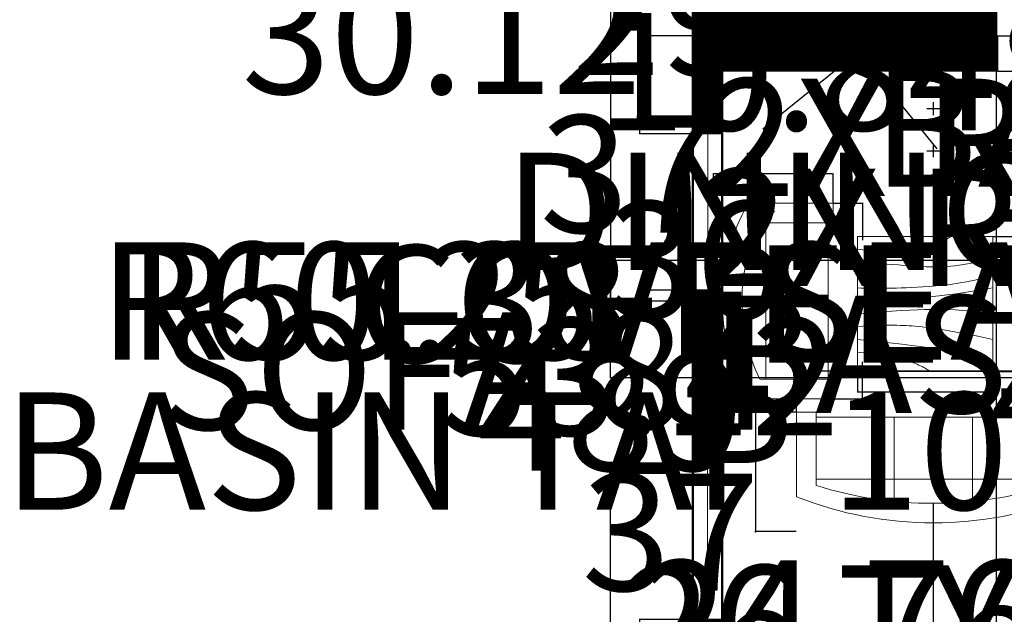
# Model space of a CAD drawing. Units: inches. Extents: x 1173 to 2157, y 515 to 1129.
# Tile 2 of 13: x 1173 to 1475, y 747 to 929. Entities that reach past the tile are written whole.
import ezdxf

# ---------------------------------------------------------------- set-up
doc = ezdxf.new("R2010")
doc.units = ezdxf.units.IN
doc.header["$MEASUREMENT"] = 0
for name, color, linetype, lineweight in [('A-ANNO-DIMS', 2, 'Continuous', 18), ('A-FLOR-CASE', 32, 'Continuous', 25), ('A-FURN', 8, 'Continuous', 18), ('A-GLAZ', 4, 'Continuous', 18), ('A-WALL', 7, 'Continuous', 50)]:
    doc.layers.add(name, color=color, linetype=linetype, lineweight=lineweight)
doc.layers.add('A-FLOR-CASE-PATT', color=28, linetype='Continuous', lineweight=13, true_color=0x301203)
doc.layers.add('A-WALL-PATT', color=22, linetype='Continuous', lineweight=13, true_color=0xca4b0c)
doc.styles.get("Standard").update_dxf_attribs({"font": 'arial.ttf'})
doc.dimstyles.get("Standard").update_dxf_attribs({"dimtxt": 36, "dimasz": 0.18, "dimexe": 0.18, "dimexo": 0.0625, "dimgap": 0.09, "dimtad": 0, "dimtih": 1, "dimtoh": 1, "dimdec": 0, "dimrnd": 72, "dimzin": 0, "dimdsep": 46, "dimlunit": 3, "dimtxsty": 'Standard', "dimcen": 2, "dimadec": 0, "dimazin": 0, "dimtfac": 1, "dimtdec": 0, "dimtofl": 0, "dimtmove": 0, "dimatfit": 3, "dimfxl": 1, "dimtolj": 1, "dimtzin": 0, "dimarcsym": 0})

# ---------------------------------------------------------------- blocks, each defined once
blk = doc.blocks.new('Table - Square Woodgrain 42 x 42 in.')
blk.add_line((0, -42), (42, -42))
for points in [[(0, -4), (1.704, -4.2172), (3.2358, -4.4188), (4.615, -4.604), (5.8615, -4.7721), (6.9951, -4.9224), (8.0357, -5.0541), (9.0031, -5.1667), (9.9171, -5.2594), (10.7951, -5.3316), (11.6445, -5.3836), (12.4702, -5.4157), (13.277, -5.4283), (14.0698, -5.4217), (14.8535, -5.3964), (15.6331, -5.3526), (16.4133, -5.2908), (17.1986, -5.2103), (17.9913, -5.1062), (18.793, -4.9727), (19.6056, -4.8038), (20.4307, -4.5937), (21.2701, -4.3365), (22.1256, -4.0262), (22.9989, -3.6571), (23.888, -3.2272), (24.7756, -2.7516), (25.6408, -2.2491), (26.4624, -1.7387), (27.2195, -1.2395), (27.891, -0.7703), (28.456, -0.3501), (28.8934, 0.002)], [(0, -42), (0, 0), (42, 0), (42, -42)], [(0, -8), (1.8203, -8.1001), (3.6741, -8.2149), (5.5411, -8.3408), (7.4011, -8.4741), (9.2339, -8.6112), (11.0193, -8.7484), (12.7371, -8.8821), (14.3671, -9.0086), (15.8954, -9.1246), (17.3337, -9.2278), (18.6997, -9.3159), (20.0116, -9.387), (21.2871, -9.4389), (22.5442, -9.4696), (23.8008, -9.477), (25.0749, -9.459), (26.3791, -9.4137), (27.7049, -9.3403), (29.0383, -9.2382), (30.3655, -9.1068), (31.6728, -8.9455), (32.9461, -8.7535), (34.1717, -8.5304), (35.3358, -8.2756), (36.4268, -7.9863), (37.443, -7.6521), (38.3849, -7.2603), (39.253, -6.7986), (40.048, -6.2542), (40.7705, -5.6147), (41.421, -4.8674), (42, -4)], [(42, -12), (39.1784, -12.8621), (36.4519, -13.5654), (33.8246, -14.1294), (31.3004, -14.5731), (28.8832, -14.9161), (26.577, -15.1775), (24.3858, -15.3768), (22.3136, -15.5332), (20.3622, -15.6632), (18.5254, -15.7718), (16.7947, -15.8612), (15.1618, -15.9338), (13.6183, -15.9916), (12.1558, -16.0369), (10.7659, -16.0718), (9.4403, -16.0987), (8.1703, -16.1191), (6.9461, -16.1325), (5.7577, -16.1377), (4.595, -16.1335), (3.4479, -16.1188), (2.3064, -16.0924), (1.1604, -16.0532), (0, -16)], [(42, -16), (37.6529, -16.7365), (33.8802, -17.329), (30.6179, -17.7961), (27.8015, -18.1561), (25.3668, -18.4275), (23.2497, -18.6288), (21.3859, -18.7785), (19.7111, -18.8949), (18.1693, -18.9939), (16.7375, -19.0795), (15.401, -19.1534), (14.1449, -19.217), (12.9544, -19.2717), (11.8148, -19.3191), (10.7113, -19.3606), (9.6291, -19.3976), (8.5534, -19.4323), (7.47, -19.4689), (6.3643, -19.5122), (5.222, -19.5672), (4.0288, -19.6386), (2.7703, -19.7313), (1.4321, -19.8501), (0, -20)], [(0, -24), (3.9243, -23.6805), (7.4766, -23.4138), (10.6891, -23.1954), (13.5943, -23.0205), (16.2247, -22.8847), (18.6125, -22.7832), (20.7903, -22.7116), (22.7903, -22.6651), (24.6563, -22.642), (26.4764, -22.6507), (28.35, -22.7024), (30.3766, -22.8084), (32.6555, -22.98), (35.2861, -23.2283), (38.3678, -23.5645), (42, -24)], [(42, -32), (37.392, -31.017), (33.4585, -30.2231), (30.1291, -29.5949), (27.3334, -29.109), (25.0009, -28.742), (23.0612, -28.4707), (21.4439, -28.2716), (20.0786, -28.1215), (18.8998, -28.0002), (17.8609, -27.9014), (16.9206, -27.8219), (16.0371, -27.7588), (15.1691, -27.709), (14.2748, -27.6693), (13.3128, -27.6368), (12.2415, -27.6083), (11.0295, -27.5824), (9.6867, -27.5643), (8.233, -27.5608), (6.6884, -27.5787), (5.0728, -27.6248), (3.4062, -27.7058), (1.7086, -27.8286), (0, -28)], [(0, -32), (5.4026, -32.5358), (9.9494, -33.019), (13.7424, -33.4553), (16.8834, -33.8505), (19.4743, -34.2106), (21.6171, -34.5413), (23.4136, -34.8486), (24.9657, -35.1382), (26.3614, -35.4156), (27.6332, -35.6841), (28.7995, -35.9467), (29.8788, -36.2064), (30.8897, -36.4661), (31.8507, -36.7288), (32.7802, -36.9973), (33.6968, -37.2747), (34.6175, -37.5635), (35.5531, -37.8651), (36.5128, -38.1805), (37.506, -38.5108), (38.5421, -38.8568), (39.6302, -39.2197), (40.7797, -39.6004), (42, -40)], [(0, -36), (3.0098, -36.2857), (5.5354, -36.5643), (7.6368, -36.8359), (9.374, -37.1009), (10.807, -37.3597), (11.9957, -37.6126), (13.0002, -37.8599), (13.8804, -38.102), (14.6874, -38.3393), (15.4365, -38.5729), (16.1338, -38.8041), (16.7858, -39.0341), (17.3987, -39.264), (17.9787, -39.4952), (18.5322, -39.7288), (19.0655, -39.9662), (19.5832, -40.2081), (20.0842, -40.4544), (20.5657, -40.7046), (21.0249, -40.9581), (21.459, -41.2144), (21.8653, -41.4731), (22.2409, -41.7335), (22.5831, -41.9951)]]:
    blk.add_lwpolyline(points)
blk = doc.blocks.new('Sofa - Roundback Loveseat 5 ft.')
for p, q in [((0, -32.44198), (0, -5.99998)), ((-24, -33.99998), (-24, -11.46958)), ((24.00004, -33.99998), (24.00004, -11.46958)), ((-23.9998, -13.38178), (23.99986, -13.38178)), ((-24, -32.44198), (24.00004, -32.44198))]:
    blk.add_line(p, q)
for points in [[(-24, -33.99998), (-30, -33.99998), (-30, -7.99998)], [(30.00004, -7.99998), (30.00004, -33.99998), (24.00004, -33.99998)]]:
    blk.add_lwpolyline(points)
for centre, radius, start, end in [((0, -60.24998), 60.24998, 60.13715, 119.8628), ((0, -61.38438), 55.38444, 64.32083, 115.6792)]:
    blk.add_arc(centre, radius, start, end)
blk = doc.blocks.new('Sofa - Roundback 7 ft.')
for p, q in [((-12.00002, -32.4421), (-12.00003, -6.5971)), ((11.99997, -32.4421), (11.99998, -6.5971)), ((-36.000027, -34), (-36.000027, -11.4696)), ((35.99998, -34), (35.99998, -11.4696)), ((-35.999844, -13.3819), (35.9998, -13.3819)), ((-36.000027, -32.4421), (35.99998, -32.4421))]:
    blk.add_line(p, q)
for points in [[(-36.000027, -34), (-42.000027, -34), (-42.000027, -8)], [(41.99998, -8), (41.99998, -34), (35.99998, -34)]]:
    blk.add_lwpolyline(points)
for centre, radius, start, end in [((0, -114.25), 114.25, 68.43141, 111.5686), ((-0.00001, -127.1968), 121.1968, 72.72033, 107.2797)]:
    blk.add_arc(centre, radius, start, end)
blk = doc.blocks.new('WIN-48X9')
blk.add_line((48, 4.5), (0, 4.5))
blk.add_lwpolyline([(0, 9), (48, 9), (48, 0), (0, 0)], close=True)
blk = doc.blocks.new('*D30')
at = {"layer": 'A-ANNO-DIMS', "color": 0, "lineweight": -2, "transparency": 16777216}
for p, q in [((1555.97, 736.03), (1563.78, 736.03)), ((1563.6, 735.85), (1563.6, 729.12)), ((1563.6, 684.97), (1563.6, 691.71)), ((1555.97, 684.79), (1563.78, 684.79))]:
    blk.add_line(p, q, dxfattribs=at)
at = {"layer": 'A-ANNO-DIMS', "color": 0, "transparency": 16777216}
for points in [[(1563.57, 735.85), (1563.63, 735.85), (1563.6, 736.03)], [(1563.57, 684.97), (1563.63, 684.97), (1563.6, 684.79)]]:
    blk.add_solid(points, dxfattribs=at)
at = {"layer": 'Defpoints', "color": 0, "transparency": 16777216}
for p in [(1555.91, 736.03), (1563.6, 736.03), (1555.91, 684.79)]:
    blk.add_point(p, dxfattribs=at)
at = {"layer": 'A-ANNO-DIMS', "color": 0, "transparency": 16777216, "insert": (1563.6, 710.41), "char_height": 36, "attachment_point": 5}
blk.add_mtext('\\A1;DESK 51 TYP.', dxfattribs=at)
blk = doc.blocks.new('*D31')
at = {"layer": 'A-ANNO-DIMS', "color": 0, "lineweight": -2, "transparency": 16777216}
for p, q in [((1529.44, 743.72), (1529.26, 743.72)), ((1529.44, 736.09), (1529.44, 743.9)), ((1555.73, 743.72), (1529.62, 743.72)), ((1555.91, 736.09), (1555.91, 743.9))]:
    blk.add_line(p, q, dxfattribs=at)
at = {"layer": 'A-ANNO-DIMS', "color": 0, "transparency": 16777216}
for points in [[(1529.62, 743.75), (1529.62, 743.69), (1529.44, 743.72)], [(1555.73, 743.75), (1555.73, 743.69), (1555.91, 743.72)]]:
    blk.add_solid(points, dxfattribs=at)
at = {"layer": 'Defpoints', "color": 0, "transparency": 16777216}
for p in [(1529.44, 743.72), (1529.44, 736.03), (1555.91, 736.03)]:
    blk.add_point(p, dxfattribs=at)
at = {"layer": 'A-ANNO-DIMS', "color": 0, "transparency": 16777216, "insert": (1441.24, 743.72), "char_height": 36, "attachment_point": 5}
blk.add_mtext('\\A1;26 TYP.', dxfattribs=at)
blk = doc.blocks.new('*D36')
at = {"layer": 'A-ANNO-DIMS', "color": 0, "lineweight": -2, "transparency": 16777216}
for p, q in [((1497.87, 905.02), (1487.37, 905.02)), ((1487.55, 904.84), (1487.55, 889.09)), ((1487.55, 835.93), (1487.55, 851.68)), ((1497.87, 835.75), (1487.37, 835.75))]:
    blk.add_line(p, q, dxfattribs=at)
at = {"layer": 'A-ANNO-DIMS', "color": 0, "transparency": 16777216}
for points in [[(1487.52, 904.84), (1487.58, 904.84), (1487.55, 905.02)], [(1487.52, 835.93), (1487.58, 835.93), (1487.55, 835.75)]]:
    blk.add_solid(points, dxfattribs=at)
at = {"layer": 'Defpoints', "color": 0, "transparency": 16777216}
for p in [(1497.94, 905.02), (1487.55, 835.75), (1497.94, 835.75)]:
    blk.add_point(p, dxfattribs=at)
at = {"layer": 'A-ANNO-DIMS', "color": 0, "transparency": 16777216, "insert": (1487.55, 870.38), "char_height": 36, "attachment_point": 5}
blk.add_mtext('\\A1;DINING SET 69', dxfattribs=at)
blk = doc.blocks.new('*D38')
at = {"layer": 'A-ANNO-DIMS', "color": 0, "lineweight": -2, "transparency": 16777216}
for p, q in [((1471.69, 862.7), (1478.04, 862.7)), ((1477.86, 862.52), (1477.86, 860.65)), ((1477.86, 821.35), (1477.86, 823.22)), ((1471.69, 821.17), (1478.04, 821.17))]:
    blk.add_line(p, q, dxfattribs=at)
at = {"layer": 'A-ANNO-DIMS', "color": 0, "transparency": 16777216}
for points in [[(1477.83, 862.52), (1477.89, 862.52), (1477.86, 862.7)], [(1477.83, 821.35), (1477.89, 821.35), (1477.86, 821.17)]]:
    blk.add_solid(points, dxfattribs=at)
at = {"layer": 'Defpoints', "color": 0, "transparency": 16777216}
for p in [(1471.63, 862.7), (1477.86, 862.7), (1471.63, 821.17)]:
    blk.add_point(p, dxfattribs=at)
at = {"layer": 'A-ANNO-DIMS', "color": 0, "transparency": 16777216, "insert": (1477.86, 841.93), "char_height": 36, "attachment_point": 5}
blk.add_mtext('\\A1;COFFEE TABLE 42', dxfattribs=at)
blk = doc.blocks.new('*D39')
at = {"layer": 'A-ANNO-DIMS', "color": 0, "lineweight": -2, "transparency": 16777216}
for p, q in [((1430.11, 821.11), (1430.11, 814.76)), ((1471.63, 821.11), (1471.63, 814.76)), ((1430.29, 814.94), (1471.45, 814.94)), ((1471.63, 814.94), (1471.81, 814.94))]:
    blk.add_line(p, q, dxfattribs=at)
at = {"layer": 'A-ANNO-DIMS', "color": 0, "transparency": 16777216}
for points in [[(1430.29, 814.97), (1430.29, 814.91), (1430.11, 814.94)], [(1471.45, 814.97), (1471.45, 814.91), (1471.63, 814.94)]]:
    blk.add_solid(points, dxfattribs=at)
at = {"layer": 'Defpoints', "color": 0, "transparency": 16777216}
for p in [(1430.11, 821.17), (1471.63, 821.17), (1471.63, 814.94)]:
    blk.add_point(p, dxfattribs=at)
at = {"layer": 'A-ANNO-DIMS', "color": 0, "transparency": 16777216, "insert": (1498.22, 814.94), "char_height": 36, "attachment_point": 5}
blk.add_mtext('\\A1;42', dxfattribs=at)
blk = doc.blocks.new('*D40')
at = {"layer": 'A-ANNO-DIMS', "color": 0, "lineweight": -2, "transparency": 16777216}
for p, q in [((1422.73, 872.86), (1431.84, 872.86)), ((1431.66, 872.68), (1431.66, 861.58)), ((1431.66, 813.04), (1431.66, 824.15)), ((1422.73, 812.86), (1431.84, 812.86))]:
    blk.add_line(p, q, dxfattribs=at)
at = {"layer": 'A-ANNO-DIMS', "color": 0, "transparency": 16777216}
for points in [[(1431.63, 872.68), (1431.69, 872.68), (1431.66, 872.86)], [(1431.63, 813.04), (1431.69, 813.04), (1431.66, 812.86)]]:
    blk.add_solid(points, dxfattribs=at)
at = {"layer": 'Defpoints', "color": 0, "transparency": 16777216}
for p in [(1422.66, 872.86), (1431.66, 872.86), (1422.66, 812.86)]:
    blk.add_point(p, dxfattribs=at)
at = {"layer": 'A-ANNO-DIMS', "color": 0, "transparency": 16777216, "insert": (1431.66, 842.86), "char_height": 36, "attachment_point": 5}
blk.add_mtext('\\A1;LOVESEAT 60', dxfattribs=at)
blk = doc.blocks.new('*D41')
at = {"layer": 'A-ANNO-DIMS', "color": 0, "lineweight": -2, "transparency": 16777216}
for p, q in [((1386, 872.92), (1386, 882.04)), ((1422.66, 872.92), (1422.66, 882.04)), ((1386, 881.86), (1385.82, 881.86)), ((1422.48, 881.86), (1386.18, 881.86))]:
    blk.add_line(p, q, dxfattribs=at)
at = {"layer": 'A-ANNO-DIMS', "color": 0, "transparency": 16777216}
for points in [[(1386.18, 881.89), (1386.18, 881.83), (1386, 881.86)], [(1422.48, 881.89), (1422.48, 881.83), (1422.66, 881.86)]]:
    blk.add_solid(points, dxfattribs=at)
at = {"layer": 'Defpoints', "color": 0, "transparency": 16777216}
for p in [(1386, 881.86), (1386, 872.86), (1422.66, 872.86)]:
    blk.add_point(p, dxfattribs=at)
at = {"layer": 'A-ANNO-DIMS', "color": 0, "transparency": 16777216, "insert": (1359.95, 881.86), "char_height": 36, "attachment_point": 5}
blk.add_mtext('\\A1;37', dxfattribs=at)
blk = doc.blocks.new('*D42')
at = {"layer": 'A-ANNO-DIMS', "color": 0, "lineweight": -2, "transparency": 16777216}
for p, q in [((1411.43, 808.8), (1411.43, 821.52)), ((1495.43, 808.8), (1495.43, 821.52)), ((1411.43, 821.34), (1411.25, 821.34)), ((1495.25, 821.34), (1411.61, 821.34))]:
    blk.add_line(p, q, dxfattribs=at)
at = {"layer": 'A-ANNO-DIMS', "color": 0, "transparency": 16777216}
for points in [[(1411.61, 821.37), (1411.61, 821.31), (1411.43, 821.34)], [(1495.25, 821.37), (1495.25, 821.31), (1495.43, 821.34)]]:
    blk.add_solid(points, dxfattribs=at)
at = {"layer": 'Defpoints', "color": 0, "transparency": 16777216}
for p in [(1411.43, 821.34), (1411.43, 808.74), (1495.43, 808.74)]:
    blk.add_point(p, dxfattribs=at)
at = {"layer": 'A-ANNO-DIMS', "color": 0, "transparency": 16777216, "insert": (1310.09, 821.34), "char_height": 36, "attachment_point": 5}
blk.add_mtext('\\A1;SOFA 84', dxfattribs=at)
blk = doc.blocks.new('*D43')
at = {"layer": 'A-ANNO-DIMS', "color": 0, "lineweight": -2, "transparency": 16777216}
for p, q in [((1411.37, 808.74), (1398.65, 808.74)), ((1398.83, 808.56), (1398.83, 772.25)), ((1411.37, 772.07), (1398.65, 772.07)), ((1398.83, 771.89), (1398.65, 771.89)), ((1398.83, 772.07), (1398.83, 771.89))]:
    blk.add_line(p, q, dxfattribs=at)
at = {"layer": 'A-ANNO-DIMS', "color": 0, "transparency": 16777216}
for points in [[(1398.8, 808.56), (1398.86, 808.56), (1398.83, 808.74)], [(1398.8, 772.25), (1398.86, 772.25), (1398.83, 772.07)]]:
    blk.add_solid(points, dxfattribs=at)
at = {"layer": 'Defpoints', "color": 0, "transparency": 16777216}
for p in [(1411.43, 808.74), (1398.83, 772.07), (1411.43, 772.07)]:
    blk.add_point(p, dxfattribs=at)
at = {"layer": 'A-ANNO-DIMS', "color": 0, "transparency": 16777216, "insert": (1372.79, 771.89), "char_height": 36, "attachment_point": 5}
blk.add_mtext('\\A1;37', dxfattribs=at)
blk = doc.blocks.new('*D46')
at = {"layer": 'A-ANNO-DIMS', "color": 0, "lineweight": -2, "transparency": 16777216}
for p, q in [((1648.72, 912.09), (1646.2, 912.17)), ((1646.37, 911.98), (1645.86, 896.32)), ((1645.85, 895.96), (1645.67, 895.96)), ((1648.2, 896.07), (1645.68, 896.15)), ((1645.86, 896.14), (1645.85, 895.96))]:
    blk.add_line(p, q, dxfattribs=at)
at = {"layer": 'A-ANNO-DIMS', "color": 0, "transparency": 16777216}
for points in [[(1646.34, 911.99), (1646.4, 911.98), (1646.38, 912.16)], [(1645.83, 896.32), (1645.89, 896.32), (1645.86, 896.14)]]:
    blk.add_solid(points, dxfattribs=at)
at = {"layer": 'Defpoints', "color": 0, "transparency": 16777216}
for p in [(1648.78, 912.09), (1645.86, 896.14), (1648.26, 896.06)]:
    blk.add_point(p, dxfattribs=at)
at = {"layer": 'A-ANNO-DIMS', "color": 0, "transparency": 16777216, "insert": (1538.16, 895.96), "char_height": 36, "attachment_point": 5}
blk.add_mtext('\\A1;BASIN 16', dxfattribs=at)
blk = doc.blocks.new('*D48')
at = {"layer": 'A-ANNO-DIMS', "color": 0, "lineweight": -2, "transparency": 16777216}
for p, q in [((1592.53, 826.46), (1592.35, 826.47)), ((1592.38, 821.85), (1592.54, 826.64)), ((1623.53, 825.46), (1592.71, 826.46)), ((1623.56, 820.84), (1623.71, 825.64))]:
    blk.add_line(p, q, dxfattribs=at)
at = {"layer": 'A-ANNO-DIMS', "color": 0, "transparency": 16777216}
for points in [[(1592.71, 826.49), (1592.71, 826.43), (1592.53, 826.46)], [(1623.53, 825.49), (1623.53, 825.43), (1623.71, 825.46)]]:
    blk.add_solid(points, dxfattribs=at)
at = {"layer": 'Defpoints', "color": 0, "transparency": 16777216}
for p in [(1592.53, 826.46), (1592.38, 821.79), (1623.56, 820.78)]:
    blk.add_point(p, dxfattribs=at)
at = {"layer": 'A-ANNO-DIMS', "color": 0, "transparency": 16777216, "insert": (1488.3, 826.47), "char_height": 36, "attachment_point": 5}
blk.add_mtext('\\A1;BASIN 31', dxfattribs=at)
blk = doc.blocks.new('*D50')
at = {"layer": 'A-ANNO-DIMS', "color": 0, "lineweight": -2, "transparency": 16777216}
for p, q in [((1603.33, 798.21), (1603.33, 796.59)), ((1613.33, 798.21), (1613.33, 796.59)), ((1603.33, 796.77), (1603.15, 796.77)), ((1613.15, 796.77), (1603.51, 796.77))]:
    blk.add_line(p, q, dxfattribs=at)
at = {"layer": 'A-ANNO-DIMS', "color": 0, "transparency": 16777216}
for points in [[(1603.51, 796.8), (1603.51, 796.74), (1603.33, 796.77)], [(1613.15, 796.8), (1613.15, 796.74), (1613.33, 796.77)]]:
    blk.add_solid(points, dxfattribs=at)
at = {"layer": 'Defpoints', "color": 0, "transparency": 16777216}
for p in [(1603.33, 798.27), (1613.33, 798.27), (1603.33, 796.77)]:
    blk.add_point(p, dxfattribs=at)
at = {"layer": 'A-ANNO-DIMS', "color": 0, "transparency": 16777216, "insert": (1377.9, 796.77), "char_height": 36, "attachment_point": 5}
blk.add_mtext('\\A1;BASIN TAP 10 TYP.', dxfattribs=at)
blk = doc.blocks.new('*D51')
at = {"layer": 'A-ANNO-DIMS', "color": 0, "lineweight": -2, "transparency": 16777216}
for p, q in [((1613.4, 804.77), (1615.01, 804.77)), ((1614.83, 804.59), (1614.83, 798.45)), ((1613.4, 798.27), (1615.01, 798.27)), ((1614.83, 798.09), (1614.65, 798.09)), ((1614.83, 798.27), (1614.83, 798.09))]:
    blk.add_line(p, q, dxfattribs=at)
at = {"layer": 'A-ANNO-DIMS', "color": 0, "transparency": 16777216}
for points in [[(1614.8, 804.59), (1614.86, 804.59), (1614.83, 804.77)], [(1614.8, 798.45), (1614.86, 798.45), (1614.83, 798.27)]]:
    blk.add_solid(points, dxfattribs=at)
at = {"layer": 'Defpoints', "color": 0, "transparency": 16777216}
for p in [(1613.33, 804.77), (1613.33, 798.27), (1614.83, 798.27)]:
    blk.add_point(p, dxfattribs=at)
at = {"layer": 'A-ANNO-DIMS', "color": 0, "transparency": 16777216, "insert": (1541.08, 798.09), "char_height": 36, "attachment_point": 5}
blk.add_mtext('\\A1;7 TYP.', dxfattribs=at)
blk = doc.blocks.new('*D54')
at = {"layer": 'A-ANNO-DIMS', "color": 0, "lineweight": -2, "transparency": 16777216}
for p, q in [((1496.35, 1005.18), (1488.93, 1005.18)), ((1489.11, 1005), (1489.11, 999.54)), ((1489.11, 956.65), (1489.11, 962.11)), ((1496.35, 956.47), (1488.93, 956.47))]:
    blk.add_line(p, q, dxfattribs=at)
at = {"layer": 'A-ANNO-DIMS', "color": 0, "transparency": 16777216}
for points in [[(1489.08, 1005), (1489.14, 1005), (1489.11, 1005.18)], [(1489.08, 956.65), (1489.14, 956.65), (1489.11, 956.47)]]:
    blk.add_solid(points, dxfattribs=at)
at = {"layer": 'Defpoints', "color": 0, "transparency": 16777216}
for p in [(1496.42, 1005.18), (1489.11, 956.47), (1496.42, 956.47)]:
    blk.add_point(p, dxfattribs=at)
at = {"layer": 'A-ANNO-DIMS', "color": 0, "transparency": 16777216, "insert": (1489.11, 980.83), "char_height": 36, "attachment_point": 5}
blk.add_mtext('\\A1;WORK TABLE 49', dxfattribs=at)
blk = doc.blocks.new('*D60')
at = {"layer": 'A-ANNO-DIMS', "color": 0, "lineweight": -2, "transparency": 16777216}
for p, q in [((1396.06, 971.62), (1390.55, 971.62)), ((1390.73, 971.62), (1390.73, 971.8)), ((1390.73, 971.8), (1390.91, 971.8)), ((1390.73, 935.8), (1390.73, 971.44)), ((1396.06, 935.62), (1390.55, 935.62))]:
    blk.add_line(p, q, dxfattribs=at)
at = {"layer": 'A-ANNO-DIMS', "color": 0, "transparency": 16777216}
for points in [[(1390.7, 971.44), (1390.76, 971.44), (1390.73, 971.62)], [(1390.7, 935.8), (1390.76, 935.8), (1390.73, 935.62)]]:
    blk.add_solid(points, dxfattribs=at)
at = {"layer": 'Defpoints', "color": 0, "transparency": 16777216}
for p in [(1390.73, 971.62), (1396.13, 971.62), (1396.13, 935.62)]:
    blk.add_point(p, dxfattribs=at)
at = {"layer": 'A-ANNO-DIMS', "color": 0, "transparency": 16777216, "insert": (1517.73, 971.8), "char_height": 36, "attachment_point": 5}
blk.add_mtext('\\A1;FRIDGE 36', dxfattribs=at)
blk = doc.blocks.new('*D61')
at = {"layer": 'A-ANNO-DIMS', "color": 0, "lineweight": -2, "transparency": 16777216}
for p, q in [((1396.13, 935.56), (1396.13, 930.04)), ((1425.13, 935.56), (1425.13, 930.04)), ((1396.13, 930.22), (1395.95, 930.22)), ((1424.95, 930.22), (1396.31, 930.22))]:
    blk.add_line(p, q, dxfattribs=at)
at = {"layer": 'A-ANNO-DIMS', "color": 0, "transparency": 16777216}
for points in [[(1396.31, 930.25), (1396.31, 930.19), (1396.13, 930.22)], [(1424.95, 930.25), (1424.95, 930.19), (1425.13, 930.22)]]:
    blk.add_solid(points, dxfattribs=at)
at = {"layer": 'Defpoints', "color": 0, "transparency": 16777216}
for p in [(1396.13, 935.62), (1425.13, 935.62), (1396.13, 930.22)]:
    blk.add_point(p, dxfattribs=at)
at = {"layer": 'A-ANNO-DIMS', "color": 0, "transparency": 16777216, "insert": (1369.73, 930.22), "char_height": 36, "attachment_point": 5}
blk.add_mtext('\\A1;29', dxfattribs=at)
blk = doc.blocks.new('*D65')
at = {"layer": 'A-ANNO-DIMS', "color": 0, "lineweight": -2, "transparency": 16777216}
for p, q in [((1379.6, 1053.28), (1354.18, 1053.28)), ((1354.36, 1053.1), (1354.36, 827.25)), ((1354.36, 564.46), (1354.36, 790.31)), ((1379.6, 564.28), (1354.18, 564.28))]:
    blk.add_line(p, q, dxfattribs=at)
at = {"layer": 'A-ANNO-DIMS', "color": 0, "transparency": 16777216}
for points in [[(1354.33, 1053.1), (1354.39, 1053.1), (1354.36, 1053.28)], [(1354.33, 564.46), (1354.39, 564.46), (1354.36, 564.28)]]:
    blk.add_solid(points, dxfattribs=at)
at = {"layer": 'Defpoints', "color": 0, "transparency": 16777216}
for p in [(1354.36, 1053.28), (1379.66, 1053.28), (1379.66, 564.28)]:
    blk.add_point(p, dxfattribs=at)
at = {"layer": 'A-ANNO-DIMS', "color": 0, "transparency": 16777216, "insert": (1354.36, 808.78), "char_height": 36, "attachment_point": 5}
blk.add_mtext('\\A1;489', dxfattribs=at)
blk = doc.blocks.new('*D69')
at = {"layer": 'A-ANNO-DIMS', "color": 0, "lineweight": -2, "transparency": 16777216}
for p, q in [((1472.66, 924.22), (1472.66, 538.8)), ((1520.66, 924.22), (1520.66, 538.8)), ((1472.84, 538.98), (1520.48, 538.98)), ((1520.66, 538.98), (1520.84, 538.98))]:
    blk.add_line(p, q, dxfattribs=at)
at = {"layer": 'A-ANNO-DIMS', "color": 0, "transparency": 16777216}
for points in [[(1472.84, 539.01), (1472.84, 538.95), (1472.66, 538.98)], [(1520.48, 539.01), (1520.48, 538.95), (1520.66, 538.98)]]:
    blk.add_solid(points, dxfattribs=at)
at = {"layer": 'Defpoints', "color": 0, "transparency": 16777216}
for p in [(1472.66, 924.28), (1520.66, 924.28), (1520.66, 538.98)]:
    blk.add_point(p, dxfattribs=at)
at = {"layer": 'A-ANNO-DIMS', "color": 0, "transparency": 16777216, "insert": (1547.48, 538.98), "char_height": 36, "attachment_point": 5}
blk.add_mtext('\\A1;48', dxfattribs=at)
blk = doc.blocks.new('*D80')
at = {"layer": 'A-ANNO-DIMS', "color": 0, "lineweight": -2, "transparency": 16777216}
for p, q in [((1388.6, 745.04), (1363.18, 745.04)), ((1363.36, 745.04), (1363.36, 745.22)), ((1363.36, 745.22), (1363.54, 745.22)), ((1363.36, 720.46), (1363.36, 744.86)), ((1388.6, 720.28), (1363.18, 720.28))]:
    blk.add_line(p, q, dxfattribs=at)
at = {"layer": 'A-ANNO-DIMS', "color": 0, "transparency": 16777216}
for points in [[(1363.33, 744.86), (1363.39, 744.86), (1363.36, 745.04)], [(1363.33, 720.46), (1363.39, 720.46), (1363.36, 720.28)]]:
    blk.add_solid(points, dxfattribs=at)
at = {"layer": 'Defpoints', "color": 0, "transparency": 16777216}
for p in [(1363.36, 745.04), (1388.66, 745.04), (1388.66, 720.28)]:
    blk.add_point(p, dxfattribs=at)
at = {"layer": 'A-ANNO-DIMS', "color": 0, "transparency": 16777216, "insert": (1424.67, 745.22), "char_height": 36, "attachment_point": 5}
blk.add_mtext('\\A1;24.76', dxfattribs=at)
blk = doc.blocks.new('*D81')
at = {"layer": 'A-ANNO-DIMS', "color": 0, "lineweight": -2, "transparency": 16777216}
for p, q in [((1388.62, 846.16), (1363.2, 846.17)), ((1363.38, 845.99), (1363.37, 838.09)), ((1363.36, 793.23), (1363.36, 801.13)), ((1388.6, 793.04), (1363.18, 793.05))]:
    blk.add_line(p, q, dxfattribs=at)
at = {"layer": 'A-ANNO-DIMS', "color": 0, "transparency": 16777216}
for points in [[(1363.35, 845.99), (1363.41, 845.99), (1363.38, 846.17)], [(1363.33, 793.23), (1363.39, 793.23), (1363.36, 793.05)]]:
    blk.add_solid(points, dxfattribs=at)
at = {"layer": 'Defpoints', "color": 0, "transparency": 16777216}
for p in [(1363.38, 846.17), (1388.68, 846.16), (1388.66, 793.04)]:
    blk.add_point(p, dxfattribs=at)
at = {"layer": 'A-ANNO-DIMS', "color": 0, "transparency": 16777216, "insert": (1363.37, 819.61), "char_height": 36, "attachment_point": 5}
blk.add_mtext('\\A1;53.12', dxfattribs=at)
blk = doc.blocks.new('*D82')
at = {"layer": 'A-ANNO-DIMS', "color": 0, "lineweight": -2, "transparency": 16777216}
for p, q in [((1363.36, 924.45), (1363.18, 924.45)), ((1388.6, 924.28), (1363.18, 924.27)), ((1363.36, 924.27), (1363.36, 924.45)), ((1363.38, 894.33), (1363.36, 924.09)), ((1388.62, 894.16), (1363.2, 894.15))]:
    blk.add_line(p, q, dxfattribs=at)
at = {"layer": 'A-ANNO-DIMS', "color": 0, "transparency": 16777216}
for points in [[(1363.39, 924.09), (1363.33, 924.09), (1363.36, 924.27)], [(1363.41, 894.33), (1363.35, 894.33), (1363.38, 894.15)]]:
    blk.add_solid(points, dxfattribs=at)
at = {"layer": 'Defpoints', "color": 0, "transparency": 16777216}
for p in [(1363.36, 924.27), (1388.66, 924.28), (1388.68, 894.16)]:
    blk.add_point(p, dxfattribs=at)
at = {"layer": 'A-ANNO-DIMS', "color": 0, "transparency": 16777216, "insert": (1302.55, 924.45), "char_height": 36, "attachment_point": 5}
blk.add_mtext('\\A1;30.12', dxfattribs=at)
blk = doc.blocks.new('*D93')
at = {"layer": 'A-ANNO-DIMS', "color": 0, "lineweight": -2, "transparency": 16777216}
for p, q in [((1473.15, 924.28), (1498.57, 924.28)), ((1498.39, 924.1), (1498.39, 913.61)), ((1473.15, 913.43), (1498.57, 913.43)), ((1498.39, 913.25), (1498.21, 913.25)), ((1498.39, 913.43), (1498.39, 913.25))]:
    blk.add_line(p, q, dxfattribs=at)
at = {"layer": 'A-ANNO-DIMS', "color": 0, "transparency": 16777216}
for points in [[(1498.36, 924.1), (1498.42, 924.1), (1498.39, 924.28)], [(1498.36, 913.61), (1498.42, 913.61), (1498.39, 913.43)]]:
    blk.add_solid(points, dxfattribs=at)
at = {"layer": 'Defpoints', "color": 0, "transparency": 16777216}
for p in [(1473.08, 924.28), (1473.08, 913.43), (1498.39, 913.43)]:
    blk.add_point(p, dxfattribs=at)
at = {"layer": 'A-ANNO-DIMS', "color": 0, "transparency": 16777216, "insert": (1425.05, 913.25), "char_height": 36, "attachment_point": 5}
blk.add_mtext('\\A1;10.848', dxfattribs=at)
blk = doc.blocks.new('*D97')
at = {"layer": 'A-ANNO-DIMS', "color": 0, "lineweight": -2, "transparency": 16777216}
for p, q in [((1580.6, 855.28), (1354.18, 855.28)), ((1354.36, 855.28), (1354.36, 855.46)), ((1354.36, 855.46), (1354.54, 855.46)), ((1354.36, 819.46), (1354.36, 855.1)), ((1580.6, 819.28), (1354.18, 819.28))]:
    blk.add_line(p, q, dxfattribs=at)
at = {"layer": 'A-ANNO-DIMS', "color": 0, "transparency": 16777216}
for points in [[(1354.33, 855.1), (1354.39, 855.1), (1354.36, 855.28)], [(1354.33, 819.46), (1354.39, 819.46), (1354.36, 819.28)]]:
    blk.add_solid(points, dxfattribs=at)
at = {"layer": 'Defpoints', "color": 0, "transparency": 16777216}
for p in [(1354.36, 855.28), (1580.66, 855.28), (1580.66, 819.28)]:
    blk.add_point(p, dxfattribs=at)
at = {"layer": 'A-ANNO-DIMS', "color": 0, "transparency": 16777216, "insert": (1380.39, 855.46), "char_height": 36, "attachment_point": 5}
blk.add_mtext('\\A1;36', dxfattribs=at)
blk = doc.blocks.new('*D103')
at = {"layer": 'A-ANNO-DIMS', "color": 0, "lineweight": -2, "transparency": 16777216}
for p, q in [((1453.43, 899.94), (1453.43, 903.94)), ((1451.43, 901.94), (1455.43, 901.94)), ((1453.43, 708.02), (1453.43, 780.56)), ((1453.25, 708.02), (1453.43, 708.02))]:
    blk.add_line(p, q, dxfattribs=at)
at = {"layer": 'A-ANNO-DIMS', "color": 0, "transparency": 16777216}
blk.add_solid([(1453.4, 780.56), (1453.46, 780.56), (1453.43, 780.74)], dxfattribs=at)
at = {"layer": 'Defpoints', "color": 0, "transparency": 16777216}
for p in [(1453.43, 901.94), (1453.43, 780.74)]:
    blk.add_point(p, dxfattribs=at)
at = {"layer": 'A-ANNO-DIMS', "color": 0, "transparency": 16777216, "insert": (1375.38, 708.02), "char_height": 36, "attachment_point": 5}
blk.add_mtext('\\A1;R121.2', dxfattribs=at)
blk = doc.blocks.new('*D104')
at = {"layer": 'A-ANNO-DIMS', "color": 0, "lineweight": -2, "transparency": 16777216}
for p, q in [((1453.43, 886.99), (1453.43, 890.99)), ((1451.43, 888.99), (1455.43, 888.99)), ((1453.43, 706.19), (1453.43, 774.56)), ((1453.25, 706.19), (1453.43, 706.19))]:
    blk.add_line(p, q, dxfattribs=at)
at = {"layer": 'A-ANNO-DIMS', "color": 0, "transparency": 16777216}
blk.add_solid([(1453.4, 774.56), (1453.46, 774.56), (1453.43, 774.74)], dxfattribs=at)
at = {"layer": 'Defpoints', "color": 0, "transparency": 16777216}
for p in [(1453.43, 888.99), (1453.43, 774.74)]:
    blk.add_point(p, dxfattribs=at)
at = {"layer": 'A-ANNO-DIMS', "color": 0, "transparency": 16777216, "insert": (1361.08, 706.19), "char_height": 36, "attachment_point": 5}
blk.add_mtext('\\A1;R114.25', dxfattribs=at)
blk = doc.blocks.new('*D105')
at = {"layer": 'A-ANNO-DIMS', "color": 0, "lineweight": -2, "transparency": 16777216}
for p, q in [((1352.51, 842.86), (1388.48, 842.86)), ((1446.91, 842.86), (1450.91, 842.86)), ((1448.91, 840.86), (1448.91, 844.86))]:
    blk.add_line(p, q, dxfattribs=at)
at = {"layer": 'A-ANNO-DIMS', "color": 0, "transparency": 16777216}
blk.add_solid([(1388.48, 842.89), (1388.48, 842.83), (1388.66, 842.86)], dxfattribs=at)
at = {"layer": 'Defpoints', "color": 0, "transparency": 16777216}
for p in [(1388.66, 842.86), (1448.91, 842.86)]:
    blk.add_point(p, dxfattribs=at)
at = {"layer": 'A-ANNO-DIMS', "color": 0, "transparency": 16777216, "insert": (1274.32, 842.86), "char_height": 36, "attachment_point": 5}
blk.add_mtext('\\A1;R60.25', dxfattribs=at)
blk = doc.blocks.new('*D106')
at = {"layer": 'A-ANNO-DIMS', "color": 0, "lineweight": -2, "transparency": 16777216}
for p, q in [((1361.43, 842.86), (1394.48, 842.86)), ((1448.05, 842.86), (1452.05, 842.86)), ((1450.05, 840.86), (1450.05, 844.86))]:
    blk.add_line(p, q, dxfattribs=at)
at = {"layer": 'A-ANNO-DIMS', "color": 0, "transparency": 16777216}
blk.add_solid([(1394.48, 842.89), (1394.48, 842.83), (1394.66, 842.86)], dxfattribs=at)
at = {"layer": 'Defpoints', "color": 0, "transparency": 16777216}
for p in [(1394.66, 842.86), (1450.05, 842.86)]:
    blk.add_point(p, dxfattribs=at)
at = {"layer": 'A-ANNO-DIMS', "color": 0, "transparency": 16777216, "insert": (1283.34, 842.86), "char_height": 36, "attachment_point": 5}
blk.add_mtext('\\A1;R55.38', dxfattribs=at)
blk = doc.blocks.new('*D108')
at = {"layer": 'A-ANNO-DIMS', "color": 0, "lineweight": -2, "transparency": 16777216}
for p, q in [((1641.43, 881.4), (1641.43, 885.4)), ((1639.43, 883.4), (1643.43, 883.4)), ((1636.72, 865.51), (1638.44, 872.04)), ((1636.54, 865.51), (1636.72, 865.51))]:
    blk.add_line(p, q, dxfattribs=at)
at = {"layer": 'A-ANNO-DIMS', "color": 0, "transparency": 16777216}
blk.add_solid([(1638.41, 872.05), (1638.47, 872.04), (1638.49, 872.22)], dxfattribs=at)
at = {"layer": 'Defpoints', "color": 0, "transparency": 16777216}
for p in [(1641.43, 883.4), (1638.49, 872.22)]:
    blk.add_point(p, dxfattribs=at)
at = {"layer": 'A-ANNO-DIMS', "color": 0, "transparency": 16777216, "insert": (1505.59, 865.51), "char_height": 36, "attachment_point": 5}
blk.add_mtext('\\A1;2X R11.564', dxfattribs=at)
blk = doc.blocks.new('*D109')
at = {"layer": 'A-ANNO-DIMS', "color": 0, "lineweight": -2, "transparency": 16777216}
for p, q in [((1638.72, 893.14), (1638.9, 893.14)), ((1638.9, 893.14), (1639.74, 886.91)), ((1639.2, 876.07), (1643.2, 876.07)), ((1641.2, 874.07), (1641.2, 878.07))]:
    blk.add_line(p, q, dxfattribs=at)
at = {"layer": 'A-ANNO-DIMS', "color": 0, "transparency": 16777216}
blk.add_solid([(1639.77, 886.92), (1639.71, 886.91), (1639.77, 886.74)], dxfattribs=at)
at = {"layer": 'Defpoints', "color": 0, "transparency": 16777216}
for p in [(1639.77, 886.74), (1641.2, 876.07)]:
    blk.add_point(p, dxfattribs=at)
at = {"layer": 'A-ANNO-DIMS', "color": 0, "transparency": 16777216, "insert": (1507.71, 893.14), "char_height": 36, "attachment_point": 5}
blk.add_mtext('\\A1;2X R10.766', dxfattribs=at)

msp = doc.modelspace()

# ---------------------------------------------------------------- hatches: boundary and pattern name
at = {"layer": 'A-FLOR-CASE-PATT'}
h = msp.add_hatch(dxfattribs=at)
h.set_pattern_fill('ANSI31', color=256)
h.paths.add_polyline_path([(1473.084, 924.2805), (1388.6635, 924.2805), (1388.6635, 913.4324), (1473.084, 913.4324)])
at = {"layer": 'A-WALL-PATT'}
h = msp.add_hatch(dxfattribs=at)
h.set_pattern_fill('ANSI31', color=256)
h.paths.add_polyline_path([(1388.6635, 933.2805), (1388.6635, 1044.2805), (1413.7618, 1044.2805), (1413.7618, 1053.2805), (1379.6635, 1053.2805), (1379.6635, 894.1606), (1388.6635, 894.1606), (1388.6635, 924.2805), (1472.6635, 924.2805), (1472.6635, 933.2805)])
h.paths.add_polyline_path([(1520.6635, 1044.2805), (1520.6635, 1014.7866), (1520.6635, 1005.1794), (1520.7714, 1005.1794), (1520.7714, 956.4707), (1520.6635, 924.2805), (1529.6635, 924.2805), (1529.6635, 931.4788), (1529.6635, 1044.2805), (1530.8474, 1044.2805), (1570.9543, 1044.2805), (1570.9543, 1053.2805), (1461.7618, 1053.2805), (1461.7618, 1044.2805)])
h.paths.add_polyline_path([(1618.9543, 1053.2805), (1618.9543, 1044.2805), (1661.6635, 1044.2805), (1661.6635, 1043.7367), (1661.6635, 1032.8874), (1670.6635, 1032.8874), (1670.6635, 1053.2805)])
h.paths.add_polyline_path([(1661.6635, 933.2805), (1661.6635, 927.8377), (1661.6635, 924.2805), (1661.6635, 918.9156), (1670.6635, 918.9156), (1670.6635, 984.8874), (1661.6635, 984.8874), (1661.6635, 978.3712)])
h.paths.add_polyline_path([(1670.6635, 894.9156), (1661.6635, 894.9156), (1661.6635, 890.0349), (1661.9328, 890.0349), (1661.9328, 870.079), (1661.6635, 864.2805), (1589.6635, 864.2805), (1589.6635, 924.2805), (1625.553, 924.2805, -0.02455299), (1625.3782, 927.8377), (1625.3782, 933.2805), (1577.6635, 933.2805), (1577.6635, 924.2805), (1580.6635, 924.2805), (1580.6635, 855.2805), (1586.1062, 855.2805), (1589.6635, 855.2805), (1661.6635, 855.2805), (1661.6635, 826.5597), (1670.6635, 826.5597)])
h.paths.add_polyline_path([(1670.6635, 802.5597), (1661.6635, 802.5597), (1661.6635, 795.2805), (1589.6635, 795.2805), (1589.6635, 819.17, -0.02455299), (1586.1062, 818.9952), (1580.6635, 818.9952), (1580.6635, 795.2805), (1577.6635, 795.2805), (1577.6635, 786.2805), (1661.6635, 786.2805), (1661.6635, 778.5597), (1661.6635, 742.6973), (1670.6635, 742.6973)])
h.paths.add_polyline_path([(1661.6635, 654.2805), (1625.1498, 654.2805), (1625.1498, 645.2805), (1661.3656, 645.2805), (1661.6635, 645.2805), (1661.6635, 573.2805), (1520.6635, 573.2805), (1520.6635, 564.2805), (1670.6635, 564.2805), (1670.6635, 694.6973), (1661.6635, 694.6973)])
h.paths.add_polyline_path([(1529.4367, 733.4702, -0.06854064), (1529.6635, 734.2623), (1529.6635, 795.2805), (1520.6635, 795.2805), (1520.6635, 645.2805), (1577.1498, 645.2805), (1577.1498, 654.2805), (1529.6635, 654.2805), (1529.6635, 686.5626, -0.06854064), (1529.4367, 687.3547)])
h.paths.add_polyline_path([(1379.6635, 711.2805), (1388.6635, 711.2805), (1458.7214, 711.2805), (1458.7214, 720.2805), (1410.7214, 720.2805), (1388.6635, 720.2805), (1388.6635, 745.0427), (1379.6635, 745.0427)])
h.paths.add_polyline_path([(1388.6635, 846.1606), (1379.6635, 846.1606), (1379.6635, 793.0427), (1388.6635, 793.0427)])

# ---------------------------------------------------------------- linework, layer by layer
at = {"layer": 'A-FLOR-CASE'}
for p, q in [((1430.4532, 919.3757), (1401.1137, 895.6125)), ((1454.5626, 889.6087), (1430.4532, 919.3757))]:
    msp.add_line(p, q, dxfattribs=at)
msp.add_lwpolyline([(1388.6635, 924.2805), (1473.084, 924.2805), (1473.084, 913.4324), (1388.6635, 913.4324)], close=True, dxfattribs=at)
at = {"layer": 'A-WALL'}
for p, q in [((1472.6635, 924.2805), (1472.6635, 933.2805)), ((1472.6635, 924.2805), (1388.6635, 924.2805)), ((1388.6635, 924.2805), (1388.6635, 720.2805))]:
    msp.add_line(p, q, dxfattribs=at)
msp.add_lwpolyline([(1379.6635, 564.2805), (1670.6635, 564.2805), (1670.6635, 1053.2805), (1379.6635, 1053.2805)], close=True, dxfattribs=at)

# ---------------------------------------------------------------- block references
at = {"layer": 'A-FURN'}
for name, p, rotation in [('Sofa - Roundback Loveseat 5 ft.', (1388.6635, 842.8621), 89.99999999999999), ('Sofa - Roundback 7 ft.', (1453.4344, 774.7398), 180)]:
    msp.add_blockref(name, p, dxfattribs=dict(at, rotation=rotation))
at = {"layer": 'A-FURN', "xscale": 0.9886638635536537, "yscale": 0.9886638635536537, "zscale": 0.9886638635536537}
msp.add_blockref('Table - Square Woodgrain 42 x 42 in.', (1430.1061, 862.6936), dxfattribs=at)
at = {"layer": 'A-GLAZ'}
for p, rotation in [((1379.6784, 894.1606), 269.9999999999996), ((1379.6635, 793.0427), 269.9999999999995)]:
    msp.add_blockref('WIN-48X9', p, dxfattribs=dict(at, rotation=rotation))

# ---------------------------------------------------------------- dimensions: what is measured, and where the dimension line sits
at = {"layer": 'A-ANNO-DIMS'}
for base, p1, p2, angle, text, picture, middle in [((1489.1107, 956.4707), (1496.4171, 1005.1794), (1496.4171, 956.4707), 270, 'WORK TABLE <>', '*D54', (1489.1107, 980.8251)), ((1390.7251, 971.618), (1396.1251, 935.618), (1396.1251, 971.618), 90, 'FRIDGE <>', '*D60', (1517.7318, 971.798)), ((1487.5464, 835.7486), (1497.9367, 905.017), (1497.9367, 835.7486), 270, 'DINING SET <>', '*D36', (1487.5464, 870.3828)), ((1645.8589, 896.1412), (1648.7786, 912.0868), (1648.2623, 896.0638), 268.15447, 'BASIN <>', '*D46', (1538.1601, 895.9613)), ((1477.8589, 862.6955), (1471.63, 821.1697), (1471.63, 862.6955), 90, 'COFFEE TABLE <>', '*D38', (1477.8589, 841.9326)), ((1603.3335, 796.7679), (1613.3335, 798.2679), (1603.3335, 798.2679), 180, 'BASIN TAP <> TYP.', '*D50', (1377.9039, 796.7679)), ((1431.6634, 872.8622), (1422.6634, 812.8621), (1422.6634, 872.8622), 90, 'LOVESEAT <>', '*D40', (1431.6634, 842.8622)), ((1592.531, 826.4624), (1623.5567, 820.7814), (1592.3803, 821.786), 178.15447, 'BASIN <>', '*D48', (1488.3007, 826.4682)), ((1411.4344, 821.3398), (1495.4344, 808.7398), (1411.4344, 808.7398), 180, 'SOFA <>', '*D42', (1310.0894, 821.3398)), ((1614.8335, 798.2679), (1613.3335, 804.768), (1613.3335, 798.2679), 270, '<> TYP.', '*D51', (1541.0778, 798.0879)), ((1529.4367, 743.7181), (1555.9105, 736.0322), (1529.4367, 736.0322), 180, '<> TYP.', '*D31', (1441.2418, 743.7181)), ((1563.5964, 736.0322), (1555.9105, 684.7928), (1555.9105, 736.0322), 90, 'DESK <> TYP.', '*D30', (1563.5964, 710.4125))]:
    dim = msp.add_linear_dim(base=base, p1=p1, p2=p2, angle=angle, text=text, dimstyle='Standard', override={"dimdec": 0, "dimlfac": 1, "dimrnd": 0, "dimzin": 0, "dimdsep": 46, "dimlunit": 2}, dxfattribs=at)
    dim.commit()
    dim.dimension.update_dxf_attribs({"geometry": picture, "text_midpoint": middle})
for base, p1, p2, angle, override, picture, middle in [((1354.361, 1053.2805), (1379.6635, 564.2805), (1379.6635, 1053.2805), 90, {"dimdec": 0, "dimlfac": 1, "dimrnd": 0, "dimzin": 0, "dimdsep": 46, "dimlunit": 2}, '*D65', (1354.361, 808.7805)), ((1396.1251, 930.218), (1425.1251, 935.618), (1396.1251, 935.618), 180, {"dimdec": 0, "dimlfac": 1, "dimrnd": 0, "dimzin": 0, "dimdsep": 46, "dimlunit": 2}, '*D61', (1369.7269, 930.218)), ((1363.361, 924.268), (1388.6784, 894.1606), (1388.6635, 924.2805), 90.028445, {"dimdec": 2, "dimlfac": 1, "dimrnd": 0, "dimzin": 0, "dimdsep": 46, "dimlunit": 2}, '*D82', (1302.5465, 924.448)), ((1498.3865, 913.4324), (1473.084, 924.2805), (1473.084, 913.4324), 270, {"dimdec": 3, "dimlfac": 1, "dimrnd": 0, "dimzin": 0, "dimdsep": 46, "dimlunit": 2}, '*D93', (1425.0483, 913.2524)), ((1385.9968, 881.8622), (1422.6634, 872.8622), (1385.9968, 872.8622), 180, {"dimdec": 0, "dimlfac": 1, "dimrnd": 0, "dimzin": 0, "dimdsep": 46, "dimlunit": 2}, '*D41', (1359.9546, 881.8622)), ((1354.361, 855.2805), (1580.6635, 819.2805), (1580.6635, 855.2805), 90, {"dimdec": 0, "dimlfac": 1, "dimrnd": 0, "dimzin": 0, "dimdsep": 46, "dimlunit": 2}, '*D97', (1380.3908, 855.4605)), ((1363.3759, 846.1677), (1388.6635, 793.0427), (1388.6784, 846.1606), 89.983871, {"dimdec": 2, "dimlfac": 1, "dimrnd": 0, "dimzin": 0, "dimdsep": 46, "dimlunit": 2}, '*D81', (1363.3684, 819.6088)), ((1398.8344, 772.0731), (1411.4344, 808.7398), (1411.4344, 772.0731), 270, {"dimdec": 0, "dimlfac": 1, "dimrnd": 0, "dimzin": 0, "dimdsep": 46, "dimlunit": 2}, '*D43', (1372.7922, 771.8931)), ((1363.361, 745.0427), (1388.6635, 720.2805), (1388.6635, 745.0427), 90, {"dimdec": 2, "dimlfac": 1, "dimrnd": 0, "dimzin": 0, "dimdsep": 46, "dimlunit": 2}, '*D80', (1424.6664, 745.2227))]:
    dim = msp.add_linear_dim(base=base, p1=p1, p2=p2, angle=angle, dimstyle='Standard', override=override, dxfattribs=at)
    dim.commit()
    dim.dimension.update_dxf_attribs({"geometry": picture, "text_midpoint": middle})
for center, mpoint, picture, middle in [((1641.2, 876.0658), (1639.765, 886.7357), '*D109', (1507.7105, 893.1376)), ((1641.4252, 883.4015), (1638.487, 872.2169), '*D108', (1505.5919, 865.5062))]:
    dim = msp.add_radius_dim(center=center, mpoint=mpoint, text='2X <>', dimstyle='Standard', override={"dimdec": 3, "dimlfac": 1, "dimrnd": 0, "dimzin": 0, "dimdsep": 46, "dimlunit": 2}, dxfattribs=at)
    dim.commit()
    dim.dimension.update_dxf_attribs({"geometry": picture, "text_midpoint": middle, "dimtype": 164})
for base, p1, p2, picture, middle in [((1520.6635, 538.978), (1472.6635, 924.2805), (1520.6635, 924.2805), '*D69', (1547.4792, 538.978)), ((1471.63, 814.9408), (1430.1061, 821.1697), (1471.63, 821.1697), '*D39', (1498.2247, 814.9408))]:
    dim = msp.add_linear_dim(base=base, p1=p1, p2=p2, dimstyle='Standard', override={"dimdec": 0, "dimlfac": 1, "dimrnd": 0, "dimzin": 0, "dimdsep": 46, "dimlunit": 2}, dxfattribs=at)
    dim.commit()
    dim.dimension.update_dxf_attribs({"geometry": picture, "text_midpoint": middle})
for center, mpoint, override, picture, middle in [((1453.4344, 901.9366), (1453.434, 780.7398), {"dimdec": 1, "dimlfac": 1, "dimrnd": 0, "dimzin": 0, "dimdsep": 46, "dimlunit": 2}, '*D103', (1375.3807, 708.0217)), ((1453.4344, 888.9898), (1453.434, 774.7398), {"dimdec": 2, "dimlfac": 1, "dimrnd": 0, "dimzin": 0, "dimdsep": 46, "dimlunit": 2}, '*D104', (1361.0764, 706.1898)), ((1448.9134, 842.8621), (1388.6635, 842.862), {"dimdec": 2, "dimlfac": 1, "dimrnd": 0, "dimzin": 0, "dimdsep": 46, "dimlunit": 2}, '*D105', (1352.5135, 842.8619)), ((1450.0478, 842.8621), (1394.6634, 842.862), {"dimdec": 2, "dimlfac": 1, "dimrnd": 0, "dimzin": 0, "dimdsep": 46, "dimlunit": 2}, '*D106', (1361.4327, 842.8619))]:
    dim = msp.add_radius_dim(center=center, mpoint=mpoint, dimstyle='Standard', override=override, dxfattribs=at)
    dim.commit()
    dim.dimension.update_dxf_attribs({"geometry": picture, "text_midpoint": middle, "dimtype": 164})

doc.saveas('drawing.dxf')
